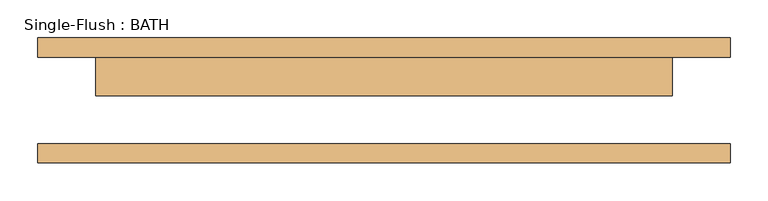
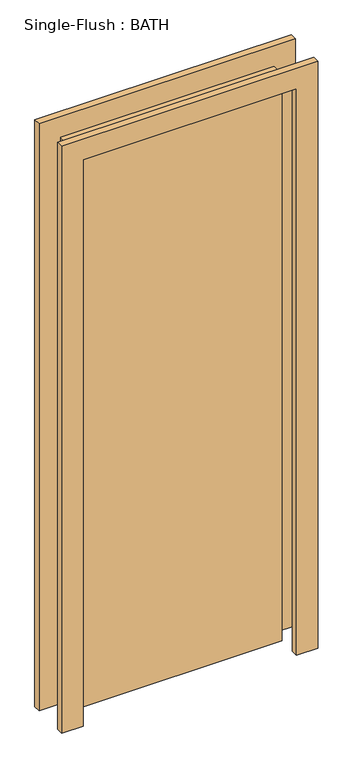
"""IFC4 building model written with IfcOpenShell, lengths in millimetres: door geometry, Single-Flush : BATH."""

from ifc_helpers import new_model, si_unit, frame, origin, origin_with_axes, place, context, project, spatial, polyline, outline, extrude, source, transform, mapped, element, save


def single_flush_bath_214872d5(model_context):
    return source(origin(), model_context, "Body", "SweptSolid", [
        extrude(outline(polyline([(2209.8, -457.2), (0.0, -457.2), (0.0, -381.0), (2133.6, -381.0), (2133.6, 381.0), (0.0, 381.0), (0.0, 457.2), (2209.8, 457.2), (2209.8, -457.2)])), frame((0.0, 57.15, 0.0), z_axis=(0.0, 1.0, 0.0), x_axis=(0.0, 0.0, 1.0)), (0.0, 0.0, 1.0), 25.4),
        extrude(outline(polyline([(2209.8, 457.2), (2209.8, -457.2), (0.0, -457.2), (0.0, -381.0), (2133.6, -381.0), (2133.6, 381.0), (0.0, 381.0), (0.0, 457.2), (2209.8, 457.2)])), frame((0.0, -82.55, 0.0), z_axis=(0.0, 1.0, 0.0), x_axis=(0.0, 0.0, 1.0)), (0.0, 0.0, 1.0), 25.4),
        extrude(outline(polyline([(381.0, 6.35), (-381.0, 6.35), (-381.0, 57.15), (381.0, 57.15), (381.0, 6.35)])), origin_with_axes(), (0.0, 0.0, 1.0), 2133.6),
    ])


if __name__ == "__main__":
    model = new_model("IFC4")
    model_context = context("Model", 3, world=origin())
    ifc_project = project(units=[si_unit("LENGTHUNIT", "METRE", prefix="MILLI")], contexts=[model_context])
    site = spatial("IfcSite", under=ifc_project)
    building = spatial("IfcBuilding", under=site)
    placement = place(None, origin())
    single_flush_bath_shape = single_flush_bath_214872d5(model_context)
    element("IfcDoor", 1, ObjectType="Single-Flush : BATH", at=placement, inside=building, context=model_context, shape_type="MappedRepresentation", body=[
        mapped(single_flush_bath_shape, transform((0.0, 0.0, 0.0), x_axis=(1.0, 0.0, 0.0), y_axis=(0.0, 1.0, 0.0), z_axis=(0.0, 0.0, 1.0))),
    ])
    save(model, "model.ifc")

# Revit data of these elements
# Type "Single-Flush : BATH"
#   Type Mark = "9"
#   Construction Type Id = "MDOOR"
#   Assembly Code = "C1020"
#   Analytic Construction = "Metal"
#   Thickness = 0' - 2"
#   Heat Transfer Coefficient (U) = 0.651978 BTU/(h·ft²·°F)
#   Height = 7' - 0"
#   Trim Projection Ext = 0' - 1"
#   Trim Projection Int = 0' - 1"
#   Trim Width = 0' - 3"
#   Width = 2' - 6"
#   Define Thermal Properties by = 1
#   Door Material = Door - Panel
#   Frame Material = Door - Frame
#   Visual Light Transmittance = 0
#   Solar Heat Gain Coefficient = 0
#   Function = (empty or 0)
#   Wall Closure = (empty or 0)
# Element 1 (IfcDoor, "Single-Flush : BATH")
#   Materials on its faces: "Door - Frame", "Door - Panel"
# Materials
#   "Door - Panel": class "Wood", colour RGB 210 159 95, transparency 0, Cost = 0
#   "Door - Frame": colour RGB 118 70 51, transparency 0, Cost = 0
